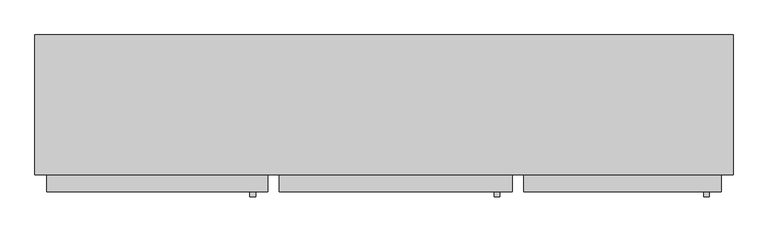
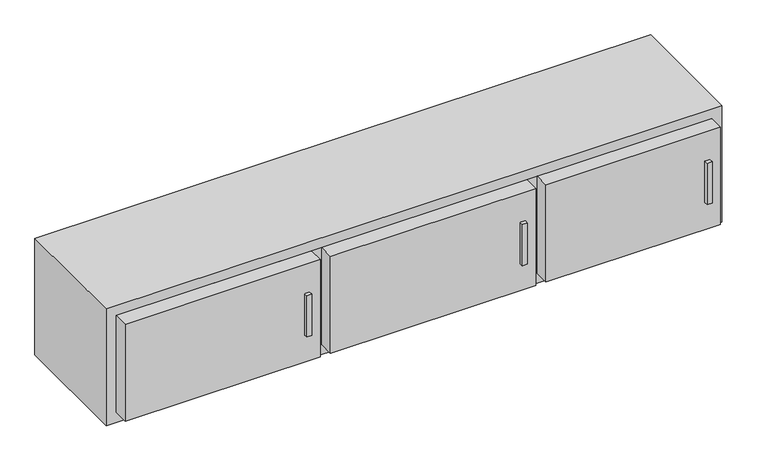
"""IFC4 building model written with IfcOpenShell, lengths in millimetres: furniture geometry."""

from ifc_helpers import new_model, si_unit, frame, origin, place, context, project, spatial, polyline, outline, extrude, faceted_brep, source, transform, mapped, element, save


def furniture_78335deb(model_context):
    return source(origin(), model_context, "Body", "SolidModel", [
        faceted_brep([(762.0, 152.4, 304.8), (-762.0, 152.4, 304.8), (-762.0, -152.4, 304.8), (762.0, -152.4, 304.8), (762.0, 152.4, 0.0), (762.0, -152.4, 0.0), (-762.0, -152.4, 0.0), (-762.0, 152.4, 0.0), (-736.6, -152.4, 279.4), (736.6, -152.4, 279.4), (736.6, -152.4, 25.4), (-736.6, -152.4, 25.4), (736.6, 116.4507166, 279.4), (-736.6, 116.4507166, 279.4), (-736.6, 116.4507166, 25.4), (736.6, 116.4507166, 25.4)], [[[0, 1, 2, 3]], [[4, 5, 6, 7]], [[1, 0, 4, 7]], [[2, 1, 7, 6]], [[3, 2, 6, 5], [8, 9, 10, 11]], [[0, 3, 5, 4]], [[12, 13, 14, 15]], [[13, 12, 9, 8]], [[14, 13, 8, 11]], [[15, 14, 11, 10]], [[12, 15, 10, 9]]]),
        extrude(outline(polyline([(-254.0, 152.4), (-228.6, 152.4), (-228.6, -152.4), (-254.0, -152.4), (-254.0, 152.4)])), frame((0.0, 0.0, 25.4), z_axis=(0.0, 0.0, 1.0), x_axis=(1.0, 0.0, 0.0)), (0.0, 0.0, 1.0), 254.0),
        extrude(outline(polyline([(279.4, 152.4), (304.8, 152.4), (304.8, -152.4), (279.4, -152.4), (279.4, 152.4)])), frame((0.0, 0.0, 25.4), z_axis=(0.0, 0.0, 1.0), x_axis=(1.0, 0.0, 0.0)), (0.0, 0.0, 1.0), 254.0),
        extrude(outline(polyline([(-736.6, -152.4), (-254.0, -152.4), (-254.0, -190.163683), (-736.6, -190.163683), (-736.6, -152.4)])), frame((0.0, 0.0, 25.4), z_axis=(0.0, 0.0, 1.0), x_axis=(1.0, 0.0, 0.0)), (0.0, 0.0, 1.0), 254.0),
        extrude(outline(polyline([(-228.6, -152.4), (279.4, -152.4), (279.4, -190.163683), (-228.6, -190.163683), (-228.6, -152.4)])), frame((0.0, 0.0, 25.4), z_axis=(0.0, 0.0, 1.0), x_axis=(1.0, 0.0, 0.0)), (0.0, 0.0, 1.0), 254.0),
        extrude(outline(polyline([(304.8, -152.4), (736.6, -152.4), (736.6, -190.163683), (304.8, -190.163683), (304.8, -152.4)])), frame((0.0, 0.0, 25.4), z_axis=(0.0, 0.0, 1.0), x_axis=(1.0, 0.0, 0.0)), (0.0, 0.0, 1.0), 254.0),
        extrude(outline(polyline([(-280.3387972, -200.4718799), (-293.0387972, -200.4718799), (-293.0387972, -190.163683), (-280.3387972, -190.163683), (-280.3387972, -200.4718799)])), frame((0.0, 0.0, 96.625737), z_axis=(0.0, 0.0, 1.0), x_axis=(1.0, 0.0, 0.0)), (0.0, 0.0, 1.0), 107.95),
        extrude(outline(polyline([(253.0612028, -200.4718799), (240.3612028, -200.4718799), (240.3612028, -190.163683), (253.0612028, -190.163683), (253.0612028, -200.4718799)])), frame((0.0, 0.0, 96.625737), z_axis=(0.0, 0.0, 1.0), x_axis=(1.0, 0.0, 0.0)), (0.0, 0.0, 1.0), 107.95),
        extrude(outline(polyline([(710.2612028, -200.4718799), (697.5612028, -200.4718799), (697.5612028, -190.163683), (710.2612028, -190.163683), (710.2612028, -200.4718799)])), frame((0.0, 0.0, 96.625737), z_axis=(0.0, 0.0, 1.0), x_axis=(1.0, 0.0, 0.0)), (0.0, 0.0, 1.0), 107.95),
    ])


if __name__ == "__main__":
    model = new_model("IFC4")
    model_context = context("Model", 3, world=origin())
    ifc_project = project(units=[si_unit("LENGTHUNIT", "METRE", prefix="MILLI")], contexts=[model_context])
    site = spatial("IfcSite", under=ifc_project)
    building = spatial("IfcBuilding", under=site)
    placement = place(None, origin())
    furniture_shape = furniture_78335deb(model_context)
    element("IfcFurniture", 1, at=placement, inside=building, context=model_context, shape_type="MappedRepresentation", body=[
        mapped(furniture_shape, transform((0.0, 0.0, 0.0), x_axis=(1.0, 0.0, 0.0), y_axis=(0.0, 1.0, 0.0), z_axis=(0.0, 0.0, 1.0))),
    ])
    save(model, "model.ifc")

# Revit data of these elements
# Type
#   Default Elevation = 0
# Element 1 (IfcFurniture)
#   Materials on its faces: "wood", "metal"
# Materials
#   "wood": class "Generic", colour RGB 173 132 96, transparency 0, Cost = 0
#   "metal": class "Generic", colour RGB 120 120 120, transparency 0, Cost = 0
